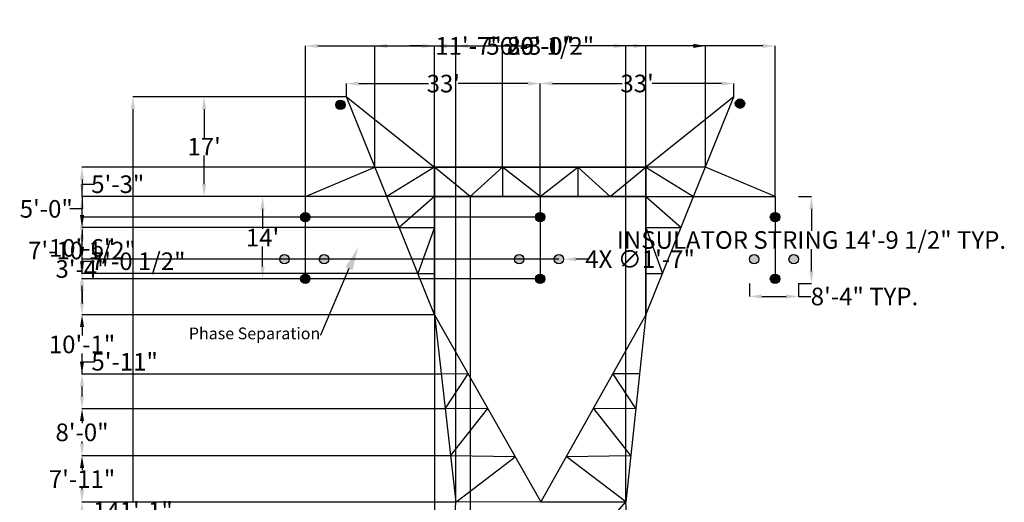
# Model space of a CAD drawing. Units: inches. Extents: x -827 to 1185, y -311 to 1858.
# Tile 2 of 2: x -827 to 1185, y 871 to 1858. Entities that reach past the tile are written whole.
import ezdxf
from ezdxf import colors
from ezdxf.entities.mleader import LeaderData, LeaderLine
from ezdxf.math import Vec2, Vec3

# ---------------------------------------------------------------- set-up
doc = ezdxf.new("R2010")
doc.units = ezdxf.units.IN
doc.header["$MEASUREMENT"] = 0
for name, color, linetype, lineweight in [('E-INSL', 3, 'Continuous', 25), ('E-SHLD', 6, 'Continuous', 25), ('S-ANNO-DIMS', 2, 'Continuous', 18), ('S-ANNO-TEXT', 7, 'Continuous', 25), ('S-TOWR', 5, 'Continuous', 30)]:
    doc.layers.add(name, color=color, linetype=linetype, lineweight=lineweight)
doc.styles.get("Standard").update_dxf_attribs({"font": 'arial.ttf'})
doc.dimstyles.get("Standard").update_dxf_attribs({"dimtxt": 36, "dimasz": 25.18, "dimexe": 0.18, "dimexo": 0.0625, "dimgap": 0.09, "dimtad": 0, "dimtih": 1, "dimtoh": 1, "dimdec": 0, "dimzin": 0, "dimdsep": 46, "dimlunit": 3, "dimtxsty": 'Standard', "dimcen": 0.09, "dimclrd": 4, "dimadec": 0, "dimazin": 0, "dimtfac": 1, "dimtdec": 0, "dimtofl": 0, "dimtmove": 0, "dimatfit": 3, "dimfxl": 1, "dimtolj": 1, "dimtzin": 0, "dimarcsym": 0})

# ---------------------------------------------------------------- blocks, each defined once
blk = doc.blocks.new('*D2')
at = {"layer": 'Defpoints', "color": 0, "transparency": 16777216}
for p in [(-159.4, 1727.6), (-159.4, 1700.6), (236.6, 1556.6)]:
    blk.add_point(p, dxfattribs=at)
at = {"layer": 'S-ANNO-DIMS', "color": 0, "lineweight": -2, "transparency": 16777216}
for p, q in [((-159.4, 1700.6), (-159.4, 1727.8)), ((-134.2, 1727.6), (8, 1727.6)), ((211.4, 1727.6), (69.2, 1727.6)), ((236.6, 1556.6), (236.6, 1727.8))]:
    blk.add_line(p, q, dxfattribs=at)
at = {"layer": 'S-ANNO-DIMS', "color": 0, "transparency": 16777216}
for points in [[(-134.2, 1731.8), (-134.2, 1723.4), (-159.4, 1727.6)], [(211.4, 1731.8), (211.4, 1723.4), (236.6, 1727.6)]]:
    blk.add_solid(points, dxfattribs=at)
at = {"layer": 'S-ANNO-DIMS', "color": 0, "transparency": 16777216, "insert": (38.6, 1727.6), "char_height": 36, "attachment_point": 5}
blk.add_mtext("\\A1;33'", dxfattribs=at)
blk = doc.blocks.new('*D3')
at = {"layer": 'Defpoints', "color": 0, "transparency": 16777216}
for p in [(236.6, 1727.8), (236.6, 1700.6), (632.6, 1700.6)]:
    blk.add_point(p, dxfattribs=at)
at = {"layer": 'S-ANNO-DIMS', "color": 0, "lineweight": -2, "transparency": 16777216}
for p, q in [((236.6, 1700.6), (236.6, 1728)), ((261.8, 1727.8), (404, 1727.8)), ((607.4, 1727.8), (465.2, 1727.8)), ((632.6, 1700.6), (632.6, 1728))]:
    blk.add_line(p, q, dxfattribs=at)
at = {"layer": 'S-ANNO-DIMS', "color": 0, "transparency": 16777216}
for points in [[(261.8, 1732), (261.8, 1723.6), (236.6, 1727.8)], [(607.4, 1732), (607.4, 1723.6), (632.6, 1727.8)]]:
    blk.add_solid(points, dxfattribs=at)
at = {"layer": 'S-ANNO-DIMS', "color": 0, "transparency": 16777216, "insert": (434.6, 1727.8), "char_height": 36, "attachment_point": 5}
blk.add_mtext("\\A1;33'", dxfattribs=at)
blk = doc.blocks.new('*D4')
at = {"layer": 'Defpoints', "color": 0, "transparency": 16777216}
for p in [(-243.4, 1496.6), (-330.9, 1328.6), (-243.4, 1328.6)]:
    blk.add_point(p, dxfattribs=at)
at = {"layer": 'S-ANNO-DIMS', "color": 0, "lineweight": -2, "transparency": 16777216}
for p, q in [((-243.5, 1496.6), (-331.1, 1496.6)), ((-330.9, 1471.4), (-330.9, 1430.7)), ((-330.9, 1353.8), (-330.9, 1394.4)), ((-243.5, 1328.6), (-331.1, 1328.6))]:
    blk.add_line(p, q, dxfattribs=at)
at = {"layer": 'S-ANNO-DIMS', "color": 0, "transparency": 16777216}
for points in [[(-335.1, 1471.4), (-326.7, 1471.4), (-330.9, 1496.6)], [(-335.1, 1353.8), (-326.7, 1353.8), (-330.9, 1328.6)]]:
    blk.add_solid(points, dxfattribs=at)
at = {"layer": 'S-ANNO-DIMS', "color": 0, "transparency": 16777216, "insert": (-330.9, 1412.6), "char_height": 36, "attachment_point": 5}
blk.add_mtext("\\A1;14'", dxfattribs=at)
blk = doc.blocks.new('*D5')
at = {"layer": 'Defpoints', "color": 0, "transparency": 16777216}
for p in [(-450.4, 1700.6), (-159.4, 1700.6), (-243.4, 1496.6)]:
    blk.add_point(p, dxfattribs=at)
at = {"layer": 'S-ANNO-DIMS', "color": 0, "lineweight": -2, "transparency": 16777216}
for p, q in [((-159.5, 1700.6), (-450.6, 1700.6)), ((-450.4, 1675.4), (-450.4, 1616.7)), ((-450.4, 1521.8), (-450.4, 1580.4)), ((-243.5, 1496.6), (-450.6, 1496.6))]:
    blk.add_line(p, q, dxfattribs=at)
at = {"layer": 'S-ANNO-DIMS', "color": 0, "transparency": 16777216}
for points in [[(-454.6, 1675.4), (-446.2, 1675.4), (-450.4, 1700.6)], [(-454.6, 1521.8), (-446.2, 1521.8), (-450.4, 1496.6)]]:
    blk.add_solid(points, dxfattribs=at)
at = {"layer": 'S-ANNO-DIMS', "color": 0, "transparency": 16777216, "insert": (-450.4, 1598.6), "char_height": 36, "attachment_point": 5}
blk.add_mtext("\\A1;17'", dxfattribs=at)
blk = doc.blocks.new('*D6')
at = {"layer": 'Defpoints', "color": 0, "transparency": 16777216}
for p in [(-159.4, 1700.6), (-595.9, 7.5), (20.6, 7.5)]:
    blk.add_point(p, dxfattribs=at)
at = {"layer": 'S-ANNO-DIMS', "color": 0, "lineweight": -2, "transparency": 16777216}
for p, q in [((-159.5, 1700.6), (-596.1, 1700.6)), ((-595.9, 1675.4), (-595.9, 872.2)), ((-595.9, 32.6), (-595.9, 835.9)), ((20.5, 7.5), (-596.1, 7.5))]:
    blk.add_line(p, q, dxfattribs=at)
at = {"layer": 'S-ANNO-DIMS', "color": 0, "transparency": 16777216}
for points in [[(-600.1, 1675.4), (-591.7, 1675.4), (-595.9, 1700.6)], [(-600.1, 32.6), (-591.7, 32.6), (-595.9, 7.5)]]:
    blk.add_solid(points, dxfattribs=at)
at = {"layer": 'S-ANNO-DIMS', "color": 0, "transparency": 16777216, "insert": (-595.9, 854), "char_height": 36, "attachment_point": 5}
blk.add_mtext('\\A1;141\'-1"', dxfattribs=at)
blk = doc.blocks.new('INSULATOR-STRING')
h = blk.add_hatch(color=256)
h.dxf.hatch_style = 1
edge = h.paths.add_edge_path()
edge.add_arc((52.4, 135.6), 9.61, 0, 360)
h = blk.add_hatch(color=256)
h.dxf.hatch_style = 1
edge = h.paths.add_edge_path()
edge.add_arc((9.6, 49.4), 9.61, 0, 360)
edge = h.paths.add_edge_path()
edge.add_arc((90.6, 49.4), 9.61, 0, 360)
h = blk.add_hatch(color=256)
h.dxf.hatch_style = 1
edge = h.paths.add_edge_path()
edge.add_arc((52.4, 9.6), 9.61, 0, 360)
blk.add_line((52.4, 177.6), (52.4, 9.6))
for centre in [(52.4, 135.6), (9.6, 49.4), (90.6, 49.4), (52.4, 9.6)]:
    blk.add_circle(centre, 9.61)
blk = doc.blocks.new('*D8')
at = {"layer": 'Defpoints', "color": 0, "transparency": 16777216}
for p in [(764.4, 1496.6), (791, 1496.6), (764.4, 1319)]:
    blk.add_point(p, dxfattribs=at)
at = {"layer": 'S-ANNO-DIMS', "color": 0, "lineweight": -2, "transparency": 16777216}
for p, q in [((764.4, 1496.6), (791.2, 1496.6)), ((764.4, 1319), (791.2, 1319))]:
    blk.add_line(p, q, dxfattribs=at)
at = {"layer": 'S-ANNO-DIMS', "color": 4, "lineweight": -2, "transparency": 16777216}
for p, q in [((791, 1471.4), (791, 1426.5)), ((791, 1344.2), (791, 1389.1))]:
    blk.add_line(p, q, dxfattribs=at)
at = {"layer": 'S-ANNO-DIMS', "color": 4, "transparency": 16777216}
for points in [[(786.8, 1471.4), (795.2, 1471.4), (791, 1496.6)], [(786.8, 1344.2), (795.2, 1344.2), (791, 1319)]]:
    blk.add_solid(points, dxfattribs=at)
at = {"layer": 'S-ANNO-DIMS', "color": 0, "transparency": 16777216, "insert": (791, 1407.8), "char_height": 36, "attachment_point": 5}
blk.add_mtext('\\A1;INSULATOR STRING 14\'-9 1/2" TYP.', dxfattribs=at)
blk = doc.blocks.new('*D9')
at = {"layer": 'Defpoints', "color": 0, "transparency": 16777216}
for p in [(664.1, 1319), (764.4, 1319), (764.4, 1292.3)]:
    blk.add_point(p, dxfattribs=at)
at = {"layer": 'S-ANNO-DIMS', "color": 0, "lineweight": -2, "transparency": 16777216}
for p, q in [((664.1, 1318.9), (664.1, 1292.2)), ((764.4, 1318.9), (764.4, 1292.2))]:
    blk.add_line(p, q, dxfattribs=at)
at = {"layer": 'S-ANNO-DIMS', "color": 4, "lineweight": -2, "transparency": 16777216}
for p, q in [((689.3, 1292.3), (739.2, 1292.3)), ((764.4, 1292.3), (789.5, 1292.3))]:
    blk.add_line(p, q, dxfattribs=at)
at = {"layer": 'S-ANNO-DIMS', "color": 4, "transparency": 16777216}
for points in [[(689.3, 1296.5), (689.3, 1288.1), (664.1, 1292.3)], [(739.2, 1296.5), (739.2, 1288.1), (764.4, 1292.3)]]:
    blk.add_solid(points, dxfattribs=at)
at = {"layer": 'S-ANNO-DIMS', "color": 0, "transparency": 16777216, "insert": (899.4, 1292.3), "char_height": 36, "attachment_point": 5}
blk.add_mtext('\\A1;8\'-4" TYP.', dxfattribs=at)
blk = doc.blocks.new('*D10')
at = {"layer": 'Defpoints', "color": 0, "transparency": 16777216}
for p in [(716.6, 1804.6), (-243.4, 1496.6), (716.6, 1496.6)]:
    blk.add_point(p, dxfattribs=at)
at = {"layer": 'S-ANNO-DIMS', "color": 0, "lineweight": -2, "transparency": 16777216}
for p, q in [((-243.4, 1496.6), (-243.4, 1804.8)), ((716.6, 1496.6), (716.6, 1804.8))]:
    blk.add_line(p, q, dxfattribs=at)
at = {"layer": 'S-ANNO-DIMS', "color": 4, "lineweight": -2, "transparency": 16777216}
for p, q in [((-218.2, 1804.6), (174.6, 1804.6)), ((691.4, 1804.6), (298.5, 1804.6))]:
    blk.add_line(p, q, dxfattribs=at)
at = {"layer": 'S-ANNO-DIMS', "color": 4, "transparency": 16777216}
for points in [[(-218.2, 1808.8), (-218.2, 1800.4), (-243.4, 1804.6)], [(691.4, 1808.8), (691.4, 1800.4), (716.6, 1804.6)]]:
    blk.add_solid(points, dxfattribs=at)
at = {"layer": 'S-ANNO-DIMS', "color": 0, "transparency": 16777216, "insert": (236.6, 1804.6), "char_height": 36, "attachment_point": 5}
blk.add_mtext('\\A1;80\'-0"', dxfattribs=at)
blk = doc.blocks.new('*D11')
at = {"layer": 'Defpoints', "color": 0, "transparency": 16777216}
for p in [(411.9, 1804.6), (63.9, 871.4), (411.9, 872.2)]:
    blk.add_point(p, dxfattribs=at)
at = {"layer": 'S-ANNO-DIMS', "color": 0, "lineweight": -2, "transparency": 16777216}
for p, q in [((63.9, 871.4), (63.9, 1804.8)), ((411.9, 872.3), (411.9, 1804.8))]:
    blk.add_line(p, q, dxfattribs=at)
at = {"layer": 'S-ANNO-DIMS', "color": 4, "lineweight": -2, "transparency": 16777216}
for p, q in [((89.1, 1804.6), (175.7, 1804.6)), ((386.7, 1804.6), (300.1, 1804.6))]:
    blk.add_line(p, q, dxfattribs=at)
at = {"layer": 'S-ANNO-DIMS', "color": 4, "transparency": 16777216}
for points in [[(89.1, 1808.8), (89.1, 1800.4), (63.9, 1804.6)], [(386.7, 1808.8), (386.7, 1800.4), (411.9, 1804.6)]]:
    blk.add_solid(points, dxfattribs=at)
at = {"layer": 'S-ANNO-DIMS', "color": 0, "transparency": 16777216, "insert": (237.9, 1804.6), "char_height": 36, "attachment_point": 5}
blk.add_mtext('\\A1;29\'-0"', dxfattribs=at)
blk = doc.blocks.new('*D12')
at = {"layer": 'Defpoints', "color": 0, "transparency": 16777216}
for p in [(452.6, 1804.6), (20.6, 1254.7), (452.6, 1254.7)]:
    blk.add_point(p, dxfattribs=at)
at = {"layer": 'S-ANNO-DIMS', "color": 0, "lineweight": -2, "transparency": 16777216}
for p, q in [((20.6, 1254.8), (20.6, 1804.8)), ((452.6, 1254.8), (452.6, 1804.8))]:
    blk.add_line(p, q, dxfattribs=at)
at = {"layer": 'S-ANNO-DIMS', "color": 4, "lineweight": -2, "transparency": 16777216}
for p, q in [((45.8, 1804.6), (174.7, 1804.6)), ((427.4, 1804.6), (298.5, 1804.6))]:
    blk.add_line(p, q, dxfattribs=at)
at = {"layer": 'S-ANNO-DIMS', "color": 4, "transparency": 16777216}
for points in [[(45.8, 1808.8), (45.8, 1800.4), (20.6, 1804.6)], [(427.4, 1808.8), (427.4, 1800.4), (452.6, 1804.6)]]:
    blk.add_solid(points, dxfattribs=at)
at = {"layer": 'S-ANNO-DIMS', "color": 0, "transparency": 16777216, "insert": (236.6, 1804.6), "char_height": 36, "attachment_point": 5}
blk.add_mtext('\\A1;36\'-0"', dxfattribs=at)
blk = doc.blocks.new('*D13')
at = {"layer": 'Defpoints', "color": 0, "transparency": 16777216}
for p in [(574.4, 1804.6), (-101.3, 1556.6), (574.4, 1556.6)]:
    blk.add_point(p, dxfattribs=at)
at = {"layer": 'S-ANNO-DIMS', "color": 0, "lineweight": -2, "transparency": 16777216}
for p, q in [((-101.3, 1556.6), (-101.3, 1804.8)), ((574.4, 1556.6), (574.4, 1804.8))]:
    blk.add_line(p, q, dxfattribs=at)
at = {"layer": 'S-ANNO-DIMS', "color": 4, "lineweight": -2, "transparency": 16777216}
for p, q in [((-76.1, 1804.6), (132.7, 1804.6)), ((549.3, 1804.6), (340.4, 1804.6))]:
    blk.add_line(p, q, dxfattribs=at)
at = {"layer": 'S-ANNO-DIMS', "color": 4, "transparency": 16777216}
for points in [[(-76.1, 1808.8), (-76.1, 1800.4), (-101.3, 1804.6)], [(549.3, 1808.8), (549.3, 1800.4), (574.4, 1804.6)]]:
    blk.add_solid(points, dxfattribs=at)
at = {"layer": 'S-ANNO-DIMS', "color": 0, "transparency": 16777216, "insert": (236.6, 1804.6), "char_height": 36, "attachment_point": 5}
blk.add_mtext('\\A1;56\'-3 1/2"', dxfattribs=at)
blk = doc.blocks.new('*D14')
at = {"layer": 'Defpoints', "color": 0, "transparency": 16777216}
for p in [(-101.3, 1556.6), (-699.9, 1496.6), (-243.4, 1496.6)]:
    blk.add_point(p, dxfattribs=at)
at = {"layer": 'S-ANNO-DIMS', "color": 0, "lineweight": -2, "transparency": 16777216}
for p, q in [((-101.3, 1556.6), (-700.1, 1556.6)), ((-243.5, 1496.6), (-700.1, 1496.6))]:
    blk.add_line(p, q, dxfattribs=at)
at = {"layer": 'S-ANNO-DIMS', "color": 4, "lineweight": -2, "transparency": 16777216}
for p, q in [((-699.9, 1531.4), (-699.9, 1521.8)), ((-699.9, 1496.6), (-699.9, 1471.4)), ((-699.9, 1471.4), (-725.1, 1471.4))]:
    blk.add_line(p, q, dxfattribs=at)
at = {"layer": 'S-ANNO-DIMS', "color": 4, "transparency": 16777216}
for points in [[(-704.1, 1531.4), (-695.7, 1531.4), (-699.9, 1556.6)], [(-704.1, 1521.8), (-695.7, 1521.8), (-699.9, 1496.6)]]:
    blk.add_solid(points, dxfattribs=at)
at = {"layer": 'S-ANNO-DIMS', "color": 0, "transparency": 16777216, "insert": (-773, 1471.4), "char_height": 36, "attachment_point": 5}
blk.add_mtext('\\A1;5\'-0"', dxfattribs=at)
blk = doc.blocks.new('*D24')
at = {"layer": 'Defpoints', "color": 0, "transparency": 16777216}
for p in [(-699.9, 871.4), (63.9, 871.4), (58.8, 770.1)]:
    blk.add_point(p, dxfattribs=at)
at = {"layer": 'S-ANNO-DIMS', "color": 0, "lineweight": -2, "transparency": 16777216}
for p, q in [((63.8, 871.4), (-700.1, 871.4)), ((58.8, 770.1), (-700.1, 770.1))]:
    blk.add_line(p, q, dxfattribs=at)
at = {"layer": 'S-ANNO-DIMS', "color": 4, "lineweight": -2, "transparency": 16777216}
for p, q in [((-699.9, 846.2), (-699.9, 839.2)), ((-699.9, 795.3), (-699.9, 802.3))]:
    blk.add_line(p, q, dxfattribs=at)
at = {"layer": 'S-ANNO-DIMS', "color": 4, "transparency": 16777216}
for points in [[(-704.1, 846.2), (-695.7, 846.2), (-699.9, 871.4)], [(-704.1, 795.3), (-695.7, 795.3), (-699.9, 770.1)]]:
    blk.add_solid(points, dxfattribs=at)
at = {"layer": 'S-ANNO-DIMS', "color": 0, "transparency": 16777216, "insert": (-699.9, 820.8), "char_height": 36, "attachment_point": 5}
blk.add_mtext('\\A1;8\'-5"', dxfattribs=at)
blk = doc.blocks.new('*D25')
at = {"layer": 'Defpoints', "color": 0, "transparency": 16777216}
for p in [(-699.9, 966.4), (53.3, 966.4), (63.9, 871.4)]:
    blk.add_point(p, dxfattribs=at)
at = {"layer": 'S-ANNO-DIMS', "color": 0, "lineweight": -2, "transparency": 16777216}
for p, q in [((53.3, 966.4), (-700.1, 966.4)), ((63.8, 871.4), (-700.1, 871.4))]:
    blk.add_line(p, q, dxfattribs=at)
at = {"layer": 'S-ANNO-DIMS', "color": 4, "lineweight": -2, "transparency": 16777216}
for p, q in [((-699.9, 941.3), (-699.9, 937.1)), ((-699.9, 896.6), (-699.9, 900.7))]:
    blk.add_line(p, q, dxfattribs=at)
at = {"layer": 'S-ANNO-DIMS', "color": 4, "transparency": 16777216}
for points in [[(-704.1, 941.3), (-695.7, 941.3), (-699.9, 966.4)], [(-704.1, 896.6), (-695.7, 896.6), (-699.9, 871.4)]]:
    blk.add_solid(points, dxfattribs=at)
at = {"layer": 'S-ANNO-DIMS', "color": 0, "transparency": 16777216, "insert": (-699.9, 918.9), "char_height": 36, "attachment_point": 5}
blk.add_mtext('\\A1;7\'-11"', dxfattribs=at)
blk = doc.blocks.new('*D26')
at = {"layer": 'Defpoints', "color": 0, "transparency": 16777216}
for p in [(-699.9, 1062.5), (42.7, 1062.5), (53.3, 966.4)]:
    blk.add_point(p, dxfattribs=at)
at = {"layer": 'S-ANNO-DIMS', "color": 0, "lineweight": -2, "transparency": 16777216}
for p, q in [((42.6, 1062.5), (-700.1, 1062.5)), ((53.3, 966.4), (-700.1, 966.4))]:
    blk.add_line(p, q, dxfattribs=at)
at = {"layer": 'S-ANNO-DIMS', "color": 4, "lineweight": -2, "transparency": 16777216}
for p, q in [((-699.9, 1037.4), (-699.9, 1033)), ((-699.9, 991.6), (-699.9, 996))]:
    blk.add_line(p, q, dxfattribs=at)
at = {"layer": 'S-ANNO-DIMS', "color": 4, "transparency": 16777216}
for points in [[(-704.1, 1037.4), (-695.7, 1037.4), (-699.9, 1062.5)], [(-704.1, 991.6), (-695.7, 991.6), (-699.9, 966.4)]]:
    blk.add_solid(points, dxfattribs=at)
at = {"layer": 'S-ANNO-DIMS', "color": 0, "transparency": 16777216, "insert": (-699.9, 1014.5), "char_height": 36, "attachment_point": 5}
blk.add_mtext('\\A1;8\'-0"', dxfattribs=at)
blk = doc.blocks.new('*D27')
at = {"layer": 'Defpoints', "color": 0, "transparency": 16777216}
for p in [(-699.9, 1133.7), (34.8, 1133.7), (42.7, 1062.5)]:
    blk.add_point(p, dxfattribs=at)
at = {"layer": 'S-ANNO-DIMS', "color": 4, "lineweight": -2, "transparency": 16777216}
for p, q in [((-699.9, 1133.7), (-699.9, 1158.8)), ((-699.9, 1158.8), (-674.7, 1158.8)), ((-699.9, 1087.7), (-699.9, 1108.5))]:
    blk.add_line(p, q, dxfattribs=at)
at = {"layer": 'S-ANNO-DIMS', "color": 0, "lineweight": -2, "transparency": 16777216}
for p, q in [((34.7, 1133.7), (-700.1, 1133.7)), ((42.6, 1062.5), (-700.1, 1062.5))]:
    blk.add_line(p, q, dxfattribs=at)
at = {"layer": 'S-ANNO-DIMS', "color": 4, "transparency": 16777216}
for points in [[(-704.1, 1108.5), (-695.7, 1108.5), (-699.9, 1133.7)], [(-704.1, 1087.7), (-695.7, 1087.7), (-699.9, 1062.5)]]:
    blk.add_solid(points, dxfattribs=at)
at = {"layer": 'S-ANNO-DIMS', "color": 0, "transparency": 16777216, "insert": (-612.8, 1158.8), "char_height": 36, "attachment_point": 5}
blk.add_mtext('\\A1;5\'-11"', dxfattribs=at)
blk = doc.blocks.new('*D28')
at = {"layer": 'Defpoints', "color": 0, "transparency": 16777216}
for p in [(-699.9, 1254.7), (20.6, 1254.7), (34.8, 1133.7)]:
    blk.add_point(p, dxfattribs=at)
at = {"layer": 'S-ANNO-DIMS', "color": 0, "lineweight": -2, "transparency": 16777216}
for p, q in [((20.5, 1254.7), (-700.1, 1254.7)), ((34.7, 1133.7), (-700.1, 1133.7))]:
    blk.add_line(p, q, dxfattribs=at)
at = {"layer": 'S-ANNO-DIMS', "color": 4, "lineweight": -2, "transparency": 16777216}
for p, q in [((-699.9, 1229.6), (-699.9, 1212.7)), ((-699.9, 1158.8), (-699.9, 1175.7))]:
    blk.add_line(p, q, dxfattribs=at)
at = {"layer": 'S-ANNO-DIMS', "color": 4, "transparency": 16777216}
for points in [[(-704.1, 1229.6), (-695.7, 1229.6), (-699.9, 1254.7)], [(-704.1, 1158.8), (-695.7, 1158.8), (-699.9, 1133.7)]]:
    blk.add_solid(points, dxfattribs=at)
at = {"layer": 'S-ANNO-DIMS', "color": 0, "transparency": 16777216, "insert": (-699.9, 1194.2), "char_height": 36, "attachment_point": 5}
blk.add_mtext('\\A1;10\'-1"', dxfattribs=at)
blk = doc.blocks.new('*D29')
at = {"layer": 'Defpoints', "color": 0, "transparency": 16777216}
for p in [(-699.9, 1339.2), (-13.5, 1339.2), (20.6, 1254.7)]:
    blk.add_point(p, dxfattribs=at)
at = {"layer": 'S-ANNO-DIMS', "color": 4, "lineweight": -2, "transparency": 16777216}
for p, q in [((-699.9, 1339.2), (-699.9, 1364.3)), ((-699.9, 1364.3), (-674.7, 1364.3)), ((-699.9, 1279.9), (-699.9, 1314))]:
    blk.add_line(p, q, dxfattribs=at)
at = {"layer": 'S-ANNO-DIMS', "color": 0, "lineweight": -2, "transparency": 16777216}
for p, q in [((-13.6, 1339.2), (-700.1, 1339.2)), ((20.5, 1254.7), (-700.1, 1254.7))]:
    blk.add_line(p, q, dxfattribs=at)
at = {"layer": 'S-ANNO-DIMS', "color": 4, "transparency": 16777216}
for points in [[(-704.1, 1314), (-695.7, 1314), (-699.9, 1339.2)], [(-704.1, 1279.9), (-695.7, 1279.9), (-699.9, 1254.7)]]:
    blk.add_solid(points, dxfattribs=at)
at = {"layer": 'S-ANNO-DIMS', "color": 0, "transparency": 16777216, "insert": (-585, 1364.3), "char_height": 36, "attachment_point": 5}
blk.add_mtext('\\A1;7\'-0 1/2"', dxfattribs=at)
blk = doc.blocks.new('*D30')
at = {"layer": 'Defpoints', "color": 0, "transparency": 16777216}
for p in [(-699.9, 1433.5), (-51.6, 1433.5), (-13.5, 1339.2)]:
    blk.add_point(p, dxfattribs=at)
at = {"layer": 'S-ANNO-DIMS', "color": 0, "lineweight": -2, "transparency": 16777216}
for p, q in [((-51.6, 1433.5), (-700.1, 1433.5)), ((-13.6, 1339.2), (-700.1, 1339.2))]:
    blk.add_line(p, q, dxfattribs=at)
at = {"layer": 'S-ANNO-DIMS', "color": 4, "lineweight": -2, "transparency": 16777216}
for p, q in [((-699.9, 1408.3), (-699.9, 1405)), ((-699.9, 1364.3), (-699.9, 1367.6))]:
    blk.add_line(p, q, dxfattribs=at)
at = {"layer": 'S-ANNO-DIMS', "color": 4, "transparency": 16777216}
for points in [[(-704.1, 1408.3), (-695.7, 1408.3), (-699.9, 1433.5)], [(-704.1, 1364.3), (-695.7, 1364.3), (-699.9, 1339.2)]]:
    blk.add_solid(points, dxfattribs=at)
at = {"layer": 'S-ANNO-DIMS', "color": 0, "transparency": 16777216, "insert": (-699.9, 1386.3), "char_height": 36, "attachment_point": 5}
blk.add_mtext('\\A1;7\'-10 1/2"', dxfattribs=at)
blk = doc.blocks.new('*D31')
at = {"layer": 'Defpoints', "color": 0, "transparency": 16777216}
for p in [(-699.9, 1496.6), (-77.1, 1496.6), (-51.6, 1433.5)]:
    blk.add_point(p, dxfattribs=at)
at = {"layer": 'S-ANNO-DIMS', "color": 4, "lineweight": -2, "transparency": 16777216}
for p, q in [((-699.9, 1496.6), (-699.9, 1521.8)), ((-699.9, 1521.8), (-674.7, 1521.8)), ((-699.9, 1458.6), (-699.9, 1471.4))]:
    blk.add_line(p, q, dxfattribs=at)
at = {"layer": 'S-ANNO-DIMS', "color": 0, "lineweight": -2, "transparency": 16777216}
for p, q in [((-77.1, 1496.6), (-700.1, 1496.6)), ((-51.6, 1433.5), (-700.1, 1433.5))]:
    blk.add_line(p, q, dxfattribs=at)
at = {"layer": 'S-ANNO-DIMS', "color": 4, "transparency": 16777216}
for points in [[(-704.1, 1471.4), (-695.7, 1471.4), (-699.9, 1496.6)], [(-704.1, 1458.6), (-695.7, 1458.6), (-699.9, 1433.5)]]:
    blk.add_solid(points, dxfattribs=at)
at = {"layer": 'S-ANNO-DIMS', "color": 0, "transparency": 16777216, "insert": (-626.8, 1521.8), "char_height": 36, "attachment_point": 5}
blk.add_mtext('\\A1;5\'-3"', dxfattribs=at)
blk = doc.blocks.new('*D32')
at = {"layer": 'Defpoints', "color": 0, "transparency": 16777216}
for p in [(159.5, 1804.6), (20.6, 1556.6), (159.5, 1556.6)]:
    blk.add_point(p, dxfattribs=at)
at = {"layer": 'S-ANNO-DIMS', "color": 4, "lineweight": -2, "transparency": 16777216}
for p, q in [((-4.6, 1804.6), (-29.8, 1804.6)), ((184.7, 1804.6), (209.8, 1804.6))]:
    blk.add_line(p, q, dxfattribs=at)
at = {"layer": 'S-ANNO-DIMS', "color": 0, "lineweight": -2, "transparency": 16777216}
for p, q in [((20.6, 1556.6), (20.6, 1804.8)), ((159.5, 1556.6), (159.5, 1804.8))]:
    blk.add_line(p, q, dxfattribs=at)
at = {"layer": 'S-ANNO-DIMS', "color": 4, "transparency": 16777216}
for points in [[(-4.6, 1808.8), (-4.6, 1800.4), (20.6, 1804.6)], [(184.7, 1808.8), (184.7, 1800.4), (159.5, 1804.6)]]:
    blk.add_solid(points, dxfattribs=at)
at = {"layer": 'S-ANNO-DIMS', "color": 0, "transparency": 16777216, "insert": (90, 1804.6), "char_height": 36, "attachment_point": 5}
blk.add_mtext('\\A1;11\'-7"', dxfattribs=at)
blk = doc.blocks.new('*D33')
at = {"layer": 'Defpoints', "color": 0, "transparency": 16777216}
for p in [(20.6, 1496.6), (93.5, 1496.6), (93.5, -249.5)]:
    blk.add_point(p, dxfattribs=at)
at = {"layer": 'S-ANNO-DIMS', "color": 0, "lineweight": -2, "transparency": 16777216}
for p, q in [((20.6, 1496.5), (20.6, -249.7)), ((93.5, 1496.5), (93.5, -249.7))]:
    blk.add_line(p, q, dxfattribs=at)
at = {"layer": 'S-ANNO-DIMS', "color": 4, "lineweight": -2, "transparency": 16777216}
for p, q in [((45.8, -249.5), (68.3, -249.5)), ((93.5, -249.5), (118.7, -249.5))]:
    blk.add_line(p, q, dxfattribs=at)
at = {"layer": 'S-ANNO-DIMS', "color": 4, "transparency": 16777216}
for points in [[(45.8, -245.3), (45.8, -253.7), (20.6, -249.5)], [(68.3, -245.3), (68.3, -253.7), (93.5, -249.5)]]:
    blk.add_solid(points, dxfattribs=at)
at = {"layer": 'S-ANNO-DIMS', "color": 0, "transparency": 16777216, "insert": (166.7, -249.5), "char_height": 36, "attachment_point": 5}
blk.add_mtext('\\A1;6\'-1"', dxfattribs=at)
blk = doc.blocks.new('*D34')
at = {"layer": 'Defpoints', "color": 0, "transparency": 16777216}
for p in [(-699.9, 1454.6), (236.6, 1454.6), (236.6, 1328.6)]:
    blk.add_point(p, dxfattribs=at)
at = {"layer": 'S-ANNO-DIMS', "color": 0, "lineweight": -2, "transparency": 16777216}
for p, q in [((236.5, 1454.6), (-700.1, 1454.6)), ((236.5, 1328.6), (-700.1, 1328.6))]:
    blk.add_line(p, q, dxfattribs=at)
at = {"layer": 'S-ANNO-DIMS', "color": 4, "lineweight": -2, "transparency": 16777216}
for p, q in [((-699.9, 1429.4), (-699.9, 1410)), ((-699.9, 1353.8), (-699.9, 1373.1))]:
    blk.add_line(p, q, dxfattribs=at)
at = {"layer": 'S-ANNO-DIMS', "color": 4, "transparency": 16777216}
for points in [[(-704.1, 1429.4), (-695.7, 1429.4), (-699.9, 1454.6)], [(-704.1, 1353.8), (-695.7, 1353.8), (-699.9, 1328.6)]]:
    blk.add_solid(points, dxfattribs=at)
at = {"layer": 'S-ANNO-DIMS', "color": 0, "transparency": 16777216, "insert": (-699.9, 1391.6), "char_height": 36, "attachment_point": 5}
blk.add_mtext('\\A1;10\'-6"', dxfattribs=at)
blk = doc.blocks.new('*D35')
at = {"layer": 'Defpoints', "color": 0, "transparency": 16777216}
for p in [(-699.9, 1368.4), (274.8, 1368.4), (236.6, 1328.6)]:
    blk.add_point(p, dxfattribs=at)
at = {"layer": 'S-ANNO-DIMS', "color": 4, "lineweight": -2, "transparency": 16777216}
for p, q in [((-699.9, 1393.5), (-699.9, 1418.7)), ((-699.9, 1303.4), (-699.9, 1278.2))]:
    blk.add_line(p, q, dxfattribs=at)
at = {"layer": 'S-ANNO-DIMS', "color": 0, "lineweight": -2, "transparency": 16777216}
for p, q in [((274.7, 1368.4), (-700.1, 1368.4)), ((236.5, 1328.6), (-700.1, 1328.6))]:
    blk.add_line(p, q, dxfattribs=at)
at = {"layer": 'S-ANNO-DIMS', "color": 4, "transparency": 16777216}
for points in [[(-704.1, 1393.5), (-695.7, 1393.5), (-699.9, 1368.4)], [(-704.1, 1303.4), (-695.7, 1303.4), (-699.9, 1328.6)]]:
    blk.add_solid(points, dxfattribs=at)
at = {"layer": 'S-ANNO-DIMS', "color": 0, "transparency": 16777216, "insert": (-699.9, 1348.5), "char_height": 36, "attachment_point": 5}
blk.add_mtext('\\A1;3\'-4"', dxfattribs=at)
blk = doc.blocks.new('*D36')
at = {"layer": 'Defpoints', "color": 0, "transparency": 16777216}
for p in [(265.2, 1368.3), (284.4, 1368.4)]:
    blk.add_point(p, dxfattribs=at)
at = {"layer": 'S-ANNO-DIMS', "color": 4, "lineweight": -2, "transparency": 16777216}
blk.add_line((334.7, 1368.6), (309.5, 1368.5), dxfattribs=at)
at = {"layer": 'S-ANNO-DIMS', "color": 0, "lineweight": -2, "transparency": 16777216}
for p, q in [((274.7, 1368.4), (274.9, 1368.4)), ((274.8, 1368.3), (274.8, 1368.4))]:
    blk.add_line(p, q, dxfattribs=at)
at = {"layer": 'S-ANNO-DIMS', "color": 4, "transparency": 16777216}
blk.add_solid([(309.5, 1372.7), (309.6, 1364.3), (284.4, 1368.4)], dxfattribs=at)
at = {"layer": 'S-ANNO-DIMS', "color": 0, "transparency": 16777216, "insert": (440.7, 1368.6), "char_height": 36, "attachment_point": 5}
blk.add_mtext('\\A1;4X ∅1\'-7"', dxfattribs=at)

msp = doc.modelspace()

# ---------------------------------------------------------------- hatches: boundary and pattern name
at = {"layer": 'E-SHLD'}
h = msp.add_hatch(color=256, dxfattribs=at)
h.dxf.hatch_style = 1
edge = h.paths.add_edge_path()
edge.add_arc((-171.61, 1684.13), 9.61, 0, 360)
h = msp.add_hatch(color=256, dxfattribs=at)
h.dxf.hatch_style = 1
edge = h.paths.add_edge_path()
edge.add_arc((644.96, 1686.54), 9.61, 0, 360)

# ---------------------------------------------------------------- linework, layer by layer
for centre in [(-171.61, 1684.13), (644.96, 1686.54)]:
    msp.add_circle(centre, 9.61, dxfattribs=at)
at = {"layer": 'S-TOWR'}
for p, q in [((159.47, 1556.58), (159.47, 1496.58)), ((236.58, 1496.58), (236.58, 1556.58)), ((313.69, 1556.58), (313.69, 1496.58)), ((20.58, 1496.58), (-51.57, 1433.46)), ((452.58, 1496.58), (524.73, 1433.46)), ((-51.57, 1433.46), (20.58, 1433.46)), ((20.58, 1433.46), (-13.5, 1339.16)), ((452.58, 1433.46), (524.73, 1433.46)), ((452.58, 1433.46), (486.66, 1339.16)), ((-13.5, 1339.16), (20.58, 1339.16)), ((452.58, 1339.16), (486.66, 1339.16)), ((20.58, 1254.75), (237.9, 872.57)), ((20.58, 1254.75), (63.91, 871.37)), ((452.58, 1254.75), (237.9, 872.57)), ((452.58, 1254.75), (411.9, 872.2)), ((20.58, 7.45), (63.91, 871.37)), ((237.9, 872.57), (63.91, 871.37)), ((237.6, 672.23), (411.9, 872.2)), ((237.9, 872.57), (411.9, 872.2)), ((452.58, 9.7), (411.9, 872.2))]:
    msp.add_line(p, q, dxfattribs=at)
for points in [[(236.58, 1496.58), (159.47, 1556.58), (93.47, 1496.58), (20.58, 1556.58), (-77.06, 1496.58), (-159.42, 1700.58), (20.58, 1556.58), (20.58, 1496.58)], [(236.58, 1496.58), (313.69, 1556.58), (379.69, 1496.58), (452.58, 1556.58), (550.22, 1496.58), (632.58, 1700.58), (452.58, 1556.58), (452.58, 1496.58)]]:
    msp.add_lwpolyline(points, close=True, dxfattribs=at)
for points in [[(236.58, 1496.58), (-243.42, 1496.58), (-101.28, 1556.58), (236.58, 1556.58), (20.58, 1556.58)], [(236.58, 1496.58), (716.58, 1496.58), (574.44, 1556.58), (236.58, 1556.58), (452.58, 1556.58)], [(20.58, 1496.58), (20.58, 1254.75), (-77.06, 1496.58)], [(452.58, 1496.58), (452.58, 1254.75), (550.22, 1496.58)], [(63.91, 871.37), (185.62, 964.62), (53.34, 966.43), (129.66, 1063.15), (42.66, 1062.55), (89.46, 1133.92), (34.75, 1133.66)], [(411.9, 872.2), (289.75, 964.87), (422.02, 967.31), (345.24, 1063.66), (432.24, 1063.48), (385.11, 1134.63), (439.81, 1134.63)]]:
    msp.add_lwpolyline(points, dxfattribs=at)

# ---------------------------------------------------------------- block references
at = {"layer": 'E-INSL'}
for p in [(-295.87, 1318.97), (184.13, 1318.97), (664.13, 1318.97)]:
    msp.add_blockref('INSULATOR-STRING', p, dxfattribs=at)

# ---------------------------------------------------------------- dimensions: what is measured, and where the dimension line sits
at = {"layer": 'S-ANNO-DIMS'}
for base, p1, p2, override, picture, middle in [((574.44, 1804.58), (-101.28, 1556.58), (574.44, 1556.58), {"dimdec": 1, "dimlfac": 1, "dimrnd": 0, "dimzin": 1, "dimdsep": 46, "dimlunit": 4, "dimfrac": 2}, '*D13', (236.58, 1804.58)), ((716.58, 1804.58), (-243.42, 1496.58), (716.58, 1496.58), {"dimdec": 1, "dimlfac": 1, "dimrnd": 0, "dimzin": 1, "dimdsep": 46, "dimlunit": 4, "dimfrac": 2}, '*D10', (236.58, 1804.58)), ((159.47, 1804.58), (20.58, 1556.58), (159.47, 1556.58), {"dimdec": 1, "dimlfac": 1, "dimrnd": 0, "dimzin": 1, "dimdsep": 46, "dimlunit": 4, "dimfrac": 2}, '*D32', (90.03, 1804.58)), ((452.58, 1804.58), (20.58, 1254.75), (452.58, 1254.75), {"dimdec": 1, "dimlfac": 1, "dimrnd": 0, "dimzin": 1, "dimdsep": 46, "dimlunit": 4, "dimfrac": 2}, '*D12', (236.58, 1804.58)), ((411.9, 1804.58), (63.91, 871.37), (411.9, 872.2), {"dimdec": 1, "dimlfac": 1, "dimrnd": 0, "dimzin": 1, "dimdsep": 46, "dimlunit": 4, "dimfrac": 2}, '*D11', (237.91, 1804.58)), ((-159.42, 1727.61), (236.58, 1556.58), (-159.42, 1700.58), {"dimclrd": 0, "dimclre": 0, "dimclrt": 0}, '*D2', (38.58, 1727.61)), ((236.58, 1727.79), (632.58, 1700.58), (236.58, 1700.58), {"dimclrd": 0, "dimclre": 0, "dimclrt": 0}, '*D3', (434.58, 1727.79)), ((93.47, -249.49), (20.58, 1496.58), (93.47, 1496.58), {"dimdec": 1, "dimlfac": 1, "dimrnd": 0, "dimzin": 1, "dimdsep": 46, "dimlunit": 4, "dimfrac": 2}, '*D33', (166.69, -249.49))]:
    dim = msp.add_linear_dim(base=base, p1=p1, p2=p2, dimstyle='Standard', override=override, dxfattribs=at)
    dim.commit()
    dim.dimension.update_dxf_attribs({"geometry": picture, "text_midpoint": middle})
for base, p1, p2, override, picture, middle in [((-595.91, 7.45), (-159.42, 1700.58), (20.58, 7.45), {"dimclrd": 0, "dimclre": 0, "dimclrt": 0}, '*D6', (-595.91, 854.01)), ((-450.43, 1700.58), (-243.42, 1496.58), (-159.42, 1700.58), {"dimclrd": 0, "dimclre": 0, "dimclrt": 0}, '*D5', (-450.43, 1598.58)), ((-699.91, 1496.58), (-101.28, 1556.58), (-243.42, 1496.58), {"dimdec": 1, "dimlfac": 1, "dimrnd": 0, "dimzin": 1, "dimdsep": 46, "dimlunit": 4, "dimfrac": 2}, '*D14', (-773.03, 1471.4)), ((-699.91, 1496.58), (-51.57, 1433.46), (-77.06, 1496.58), {"dimdec": 1, "dimlfac": 1, "dimrnd": 0, "dimzin": 1, "dimdsep": 46, "dimlunit": 4, "dimfrac": 2}, '*D31', (-626.8, 1521.76)), ((-330.94, 1328.58), (-243.42, 1496.58), (-243.42, 1328.58), {"dimclrd": 0, "dimclre": 0, "dimclrt": 0}, '*D4', (-330.94, 1412.58)), ((-699.91, 1454.58), (236.58, 1328.58), (236.58, 1454.58), {"dimdec": 1, "dimlfac": 1, "dimrnd": 0, "dimzin": 1, "dimdsep": 46, "dimlunit": 4, "dimfrac": 2}, '*D34', (-699.91, 1391.58)), ((-699.91, 1433.46), (-13.5, 1339.16), (-51.57, 1433.46), {"dimdec": 1, "dimlfac": 1, "dimrnd": 0, "dimzin": 1, "dimdsep": 46, "dimlunit": 4, "dimfrac": 2}, '*D30', (-699.91, 1386.31)), ((-699.91, 1368.35), (236.58, 1328.58), (274.76, 1368.35), {"dimdec": 1, "dimlfac": 1, "dimrnd": 0, "dimzin": 1, "dimdsep": 46, "dimlunit": 4, "dimfrac": 2}, '*D35', (-699.91, 1348.46)), ((-699.91, 1339.16), (20.58, 1254.75), (-13.5, 1339.16), {"dimdec": 1, "dimlfac": 1, "dimrnd": 0, "dimzin": 1, "dimdsep": 46, "dimlunit": 4, "dimfrac": 2}, '*D29', (-585, 1364.34)), ((-699.91, 1254.75), (34.75, 1133.66), (20.58, 1254.75), {"dimdec": 1, "dimlfac": 1, "dimrnd": 0, "dimzin": 1, "dimdsep": 46, "dimlunit": 4, "dimfrac": 2}, '*D28', (-699.91, 1194.21)), ((-699.91, 1133.66), (42.66, 1062.55), (34.75, 1133.66), {"dimdec": 1, "dimlfac": 1, "dimrnd": 0, "dimzin": 1, "dimdsep": 46, "dimlunit": 4, "dimfrac": 2}, '*D27', (-612.81, 1158.84)), ((-699.91, 1062.55), (53.34, 966.43), (42.66, 1062.55), {"dimdec": 1, "dimlfac": 1, "dimrnd": 0, "dimzin": 1, "dimdsep": 46, "dimlunit": 4, "dimfrac": 2}, '*D26', (-699.91, 1014.49)), ((-699.91, 966.43), (63.91, 871.37), (53.34, 966.43), {"dimdec": 1, "dimlfac": 1, "dimrnd": 0, "dimzin": 1, "dimdsep": 46, "dimlunit": 4, "dimfrac": 2}, '*D25', (-699.91, 918.9)), ((-699.91, 871.37), (58.83, 770.15), (63.91, 871.37), {"dimdec": 1, "dimlfac": 1, "dimrnd": 0, "dimzin": 1, "dimdsep": 46, "dimlunit": 4, "dimfrac": 2}, '*D24', (-699.91, 820.76))]:
    dim = msp.add_linear_dim(base=base, p1=p1, p2=p2, angle=90, dimstyle='Standard', override=override, dxfattribs=at)
    dim.commit()
    dim.dimension.update_dxf_attribs({"geometry": picture, "text_midpoint": middle})
dim = msp.add_linear_dim(base=(791.01, 1496.58), p1=(764.37, 1318.97), p2=(764.37, 1496.58), angle=90, text='INSULATOR STRING <> TYP.', dimstyle='Standard', override={"dimdec": 1, "dimlfac": 1, "dimrnd": 0, "dimzin": 1, "dimdsep": 46, "dimlunit": 4, "dimfrac": 2}, dxfattribs=at)
dim.commit()
dim.dimension.update_dxf_attribs({"geometry": '*D8', "text_midpoint": (791.01, 1407.77)})
dim = msp.add_diameter_dim_2p(p1=(265.16, 1368.31), p2=(284.37, 1368.4), text='4X <>', dimstyle='Standard', override={"dimdec": 1, "dimlfac": 1, "dimrnd": 0, "dimzin": 1, "dimdsep": 46, "dimlunit": 4, "dimfrac": 2}, dxfattribs=at)
dim.commit()
dim.dimension.update_dxf_attribs({"geometry": '*D36', "text_midpoint": (334.73, 1368.64)})
dim = msp.add_linear_dim(base=(764.37, 1292.33), p1=(664.13, 1318.97), p2=(764.37, 1318.97), text='<> TYP.', dimstyle='Standard', override={"dimdec": 1, "dimlfac": 1, "dimrnd": 0, "dimzin": 1, "dimdsep": 46, "dimlunit": 4, "dimfrac": 2}, dxfattribs=at)
dim.commit()
dim.dimension.update_dxf_attribs({"geometry": '*D9', "text_midpoint": (899.38, 1292.33)})

# ---------------------------------------------------------------- leaders
at = {"layer": 'S-ANNO-TEXT'}
ml = msp.add_multileader_mtext('Standard', dxfattribs=at)
ml.set_content('Phase Separation', color=6)
ml.set_leader_properties(color=1)
ml.build(insert=Vec2(0, 0))
ml.multileader.update_dxf_attribs({"dogleg_length": 0.36, "arrow_head_size": 48})
ctx = ml.context
ctx.base_point, ctx.char_height, ctx.arrow_head_size, ctx.landing_gap_size, ctx.plane_origin = Vec3(-474.72, 1213.37), 24, 48, 0.09, Vec3(-212.52, 1213.37)
ctx.text_align_type = 2
notes = []
notes.append((ctx, [(0, (1, 1, 0), (-212.52, 1213.37), (-1, 0), 0.36, [(0, [(-135.35, 1393.28)], 0, [])])]))
ctx.mtext.insert, ctx.mtext.alignment, ctx.mtext.flow_direction = Vec3(-212.97, 1228.7), 3, 5
for ctx, leaders in notes:
    for number, flags, end, landing, length, lines in leaders:
        leader = LeaderData()
        leader.index, (leader.has_last_leader_line, leader.has_dogleg_vector, leader.attachment_direction) = number, flags
        leader.last_leader_point, leader.dogleg_vector, leader.dogleg_length = Vec3(end), Vec3(landing), length
        for number, points, colour, breaks in lines:
            line = LeaderLine()
            line.index, line.vertices, line.color, line.breaks = number, Vec3.list(points), colors.encode_raw_color(colour), breaks
            leader.lines.append(line)
        ctx.leaders.append(leader)

doc.saveas('drawing.dxf')
